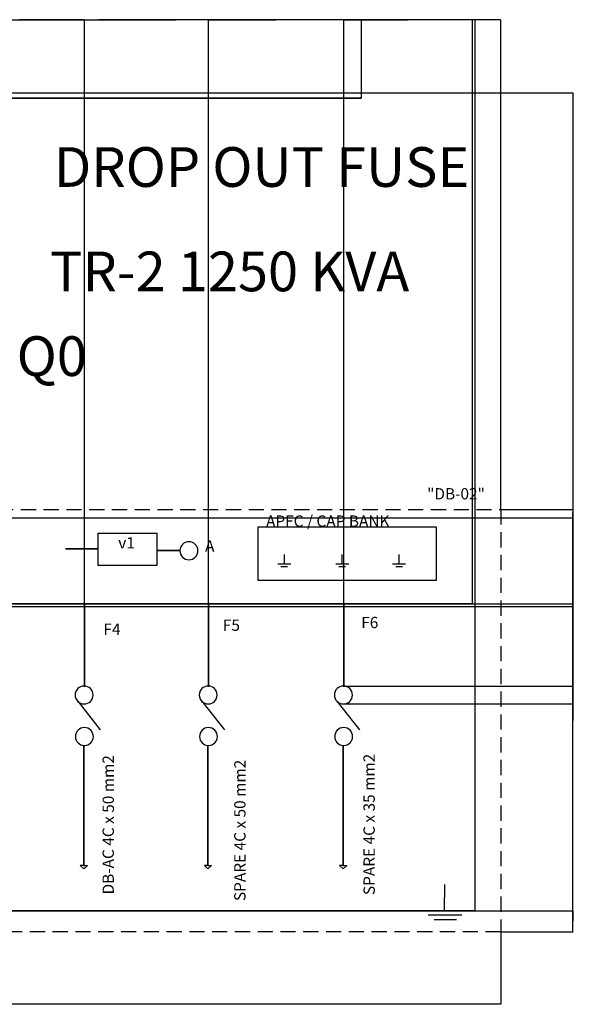
# Model space of a CAD drawing. Units: millimetres. Extents: x 1832 to 3146, y 927 to 1751.
# Tile 4 of 4: x 2683 to 3146, y 927 to 1751. Entities that reach past the tile are written whole.
import ezdxf

# ---------------------------------------------------------------- set-up
doc = ezdxf.new("R2010")
doc.units = ezdxf.units.MM
doc.header["$MEASUREMENT"] = 0
doc.linetypes.add('DASHED', pattern=[19.05, 12.7, -6.35])
doc.layers.get('0').update_dxf_attribs({"color": 2, "lineweight": 35})
doc.layers.get('0').transparency = 0.01
for name, color, linetype, lineweight in [('A-ANNO-DIMS', 2, 'Continuous', 18), ('E-ANNO-TEXT', 7, 'Continuous', 18), ('E-POWR-EQPM', 2, 'Continuous', 25), ('E-POWR-PNLS', 3, 'DASHED', 25), ('E-POWR-WIRE', 7, 'Continuous', 35)]:
    doc.layers.add(name, color=color, linetype=linetype, lineweight=lineweight)
doc.styles.get("Standard").update_dxf_attribs({"font": 'arial.ttf'})
doc.dimstyles.get("Standard").update_dxf_attribs({"dimtxt": 0.18, "dimasz": 0.18, "dimexe": 0.18, "dimexo": 0.0625, "dimgap": 0.09, "dimtad": 0, "dimtih": 1, "dimtoh": 1, "dimdec": 4, "dimzin": 0, "dimdsep": 46, "dimtxsty": 'Standard', "dimcen": 0.09, "dimadec": 0, "dimazin": 0, "dimtfac": 1, "dimtdec": 4, "dimtofl": 0, "dimtmove": 0, "dimatfit": 3, "dimfxl": 1, "dimtolj": 1, "dimtzin": 0, "dimarcsym": 0})

# ---------------------------------------------------------------- blocks, each defined once
blk = doc.blocks.new('CB-FEEDER')
blk.add_line((1982.97, 1178.23), (2001.83, 1154.39))
for points in [[(1980.83, 1183.48, 1), (1995.83, 1183.48, 1)], [(1981.05, 1148.75, 1), (1996.05, 1148.75, 1)]]:
    blk.add_lwpolyline(points, format="xyb", close=True)
blk = doc.blocks.new('CABLE-ARROW')
for p, q in [((1988.1, 1040.89), (1985.1, 1040.84)), ((1985.1, 1040.84), (1988.1, 1038.05)), ((1988.1, 1040.89), (1991.1, 1040.89)), ((1991.1, 1040.89), (1988.1, 1038.05))]:
    blk.add_line(p, q)
blk = doc.blocks.new('EARTH')
for p, q in [((2904.21, 1303.5), (2904.21, 1295.71)), ((2898.96, 1295.71), (2909.83, 1295.71)), ((2901.62, 1293.58), (2907.16, 1293.58))]:
    blk.add_line(p, q)
blk = doc.blocks.new('*D9')
at = {"layer": 'A-ANNO-DIMS', "color": 0, "lineweight": -2, "transparency": 16777216}
for p, q in [((1892.94, 1002.86), (1892.94, 927.26)), ((3085.33, 987.73), (3085.33, 927.26)), ((1893.12, 927.44), (2488.68, 927.44)), ((3085.15, 927.44), (2489.59, 927.44))]:
    blk.add_line(p, q, dxfattribs=at)
at = {"layer": 'A-ANNO-DIMS', "color": 0, "lineweight": 35, "transparency": 16777216}
for points in [[(1893.12, 927.47), (1893.12, 927.41), (1892.94, 927.44)], [(3085.15, 927.47), (3085.15, 927.41), (3085.33, 927.44)]]:
    blk.add_solid(points, dxfattribs=at)
at = {"layer": 'Defpoints', "color": 0, "lineweight": 35, "transparency": 16777216}
for p in [(1892.94, 1002.93), (3085.33, 987.79), (3085.33, 927.44)]:
    blk.add_point(p, dxfattribs=at)
at = {"layer": 'A-ANNO-DIMS', "color": 0, "transparency": 16777216, "insert": (2489.13, 927.44), "char_height": 0.18, "attachment_point": 5}
blk.add_mtext('\\A1;1192.4', dxfattribs=at)
blk = doc.blocks.new('*D10')
at = {"layer": 'A-ANNO-DIMS', "color": 0, "lineweight": -2, "transparency": 16777216}
for p, q in [((2658.48, 1689.58), (3145.86, 1689.58)), ((3145.68, 1689.4), (3145.68, 1338.87)), ((3145.68, 987.97), (3145.68, 1338.5)), ((3085.39, 987.79), (3145.86, 987.79))]:
    blk.add_line(p, q, dxfattribs=at)
at = {"layer": 'A-ANNO-DIMS', "color": 0, "lineweight": 35, "transparency": 16777216}
for points in [[(3145.65, 1689.4), (3145.71, 1689.4), (3145.68, 1689.58)], [(3145.65, 987.97), (3145.71, 987.97), (3145.68, 987.79)]]:
    blk.add_solid(points, dxfattribs=at)
at = {"layer": 'Defpoints', "color": 0, "lineweight": 35, "transparency": 16777216}
for p in [(2658.42, 1689.58), (3145.68, 1689.58), (3085.33, 987.79)]:
    blk.add_point(p, dxfattribs=at)
at = {"layer": 'A-ANNO-DIMS', "color": 0, "transparency": 16777216, "insert": (3145.68, 1338.68), "char_height": 0.18, "attachment_point": 5}
blk.add_mtext('\\A1;701.8', dxfattribs=at)
blk = doc.blocks.new('*D18')
at = {"layer": 'A-ANNO-DIMS', "color": 0, "lineweight": -2, "transparency": 16777216}
for p, q in [((2627.92, 1262.43), (2627.92, 1750.84)), ((2628.1, 1750.66), (2682.1, 1750.66)), ((2737.01, 1750.66), (2683.01, 1750.66)), ((2737.19, 1262.43), (2737.19, 1750.84))]:
    blk.add_line(p, q, dxfattribs=at)
at = {"layer": 'A-ANNO-DIMS', "color": 0, "lineweight": 35, "transparency": 16777216}
for points in [[(2628.1, 1750.69), (2628.1, 1750.63), (2627.92, 1750.66)], [(2737.01, 1750.69), (2737.01, 1750.63), (2737.19, 1750.66)]]:
    blk.add_solid(points, dxfattribs=at)
at = {"layer": 'Defpoints', "color": 0, "lineweight": 35, "transparency": 16777216}
for p in [(2737.19, 1750.66), (2627.92, 1262.37), (2737.19, 1262.37)]:
    blk.add_point(p, dxfattribs=at)
at = {"layer": 'A-ANNO-DIMS', "color": 0, "transparency": 16777216, "insert": (2682.56, 1750.66), "char_height": 0.18, "attachment_point": 5}
blk.add_mtext('\\A1;109.27', dxfattribs=at)
blk = doc.blocks.new('*D19')
at = {"layer": 'A-ANNO-DIMS', "color": 0, "lineweight": -2, "transparency": 16777216}
for p, q in [((2737.19, 1262.43), (2737.19, 1750.84)), ((2737.37, 1750.66), (2788.62, 1750.66)), ((2840.78, 1750.66), (2789.53, 1750.66)), ((2840.96, 1262.43), (2840.96, 1750.84))]:
    blk.add_line(p, q, dxfattribs=at)
at = {"layer": 'A-ANNO-DIMS', "color": 0, "lineweight": 35, "transparency": 16777216}
for points in [[(2737.37, 1750.69), (2737.37, 1750.63), (2737.19, 1750.66)], [(2840.78, 1750.69), (2840.78, 1750.63), (2840.96, 1750.66)]]:
    blk.add_solid(points, dxfattribs=at)
at = {"layer": 'Defpoints', "color": 0, "lineweight": 35, "transparency": 16777216}
for p in [(2840.96, 1750.66), (2737.19, 1262.37), (2840.96, 1262.37)]:
    blk.add_point(p, dxfattribs=at)
at = {"layer": 'A-ANNO-DIMS', "color": 0, "transparency": 16777216, "insert": (2789.08, 1750.66), "char_height": 0.18, "attachment_point": 5}
blk.add_mtext('\\A1;103.77', dxfattribs=at)
blk = doc.blocks.new('*D20')
at = {"layer": 'A-ANNO-DIMS', "color": 0, "lineweight": -2, "transparency": 16777216}
for p, q in [((2840.96, 1262.43), (2840.96, 1750.84)), ((2841.14, 1750.66), (2897.04, 1750.66)), ((2953.85, 1750.66), (2897.95, 1750.66)), ((2954.03, 1262.43), (2954.03, 1750.84))]:
    blk.add_line(p, q, dxfattribs=at)
at = {"layer": 'A-ANNO-DIMS', "color": 0, "lineweight": 35, "transparency": 16777216}
for points in [[(2841.14, 1750.69), (2841.14, 1750.63), (2840.96, 1750.66)], [(2953.85, 1750.69), (2953.85, 1750.63), (2954.03, 1750.66)]]:
    blk.add_solid(points, dxfattribs=at)
at = {"layer": 'Defpoints', "color": 0, "lineweight": 35, "transparency": 16777216}
for p in [(2954.03, 1750.66), (2840.96, 1262.37), (2954.03, 1262.37)]:
    blk.add_point(p, dxfattribs=at)
at = {"layer": 'A-ANNO-DIMS', "color": 0, "transparency": 16777216, "insert": (2897.49, 1750.66), "char_height": 0.18, "attachment_point": 5}
blk.add_mtext('\\A1;113.07', dxfattribs=at)
blk = doc.blocks.new('*D22')
at = {"layer": 'A-ANNO-DIMS', "color": 0, "lineweight": -2, "transparency": 16777216}
for p, q in [((3085.39, 1341.19), (3145.86, 1341.19)), ((3145.68, 1341.01), (3145.68, 1164.67)), ((3145.68, 987.97), (3145.68, 1164.31)), ((3085.39, 987.79), (3145.86, 987.79))]:
    blk.add_line(p, q, dxfattribs=at)
at = {"layer": 'A-ANNO-DIMS', "color": 0, "lineweight": 35, "transparency": 16777216}
for points in [[(3145.65, 1341.01), (3145.71, 1341.01), (3145.68, 1341.19)], [(3145.65, 987.97), (3145.71, 987.97), (3145.68, 987.79)]]:
    blk.add_solid(points, dxfattribs=at)
at = {"layer": 'Defpoints', "color": 0, "lineweight": 35, "transparency": 16777216}
for p in [(3085.33, 1341.19), (3145.68, 1341.19), (3085.33, 987.79)]:
    blk.add_point(p, dxfattribs=at)
at = {"layer": 'A-ANNO-DIMS', "color": 0, "transparency": 16777216, "insert": (3145.68, 1164.49), "char_height": 0.18, "attachment_point": 5}
blk.add_mtext('\\A1;353.4', dxfattribs=at)
blk = doc.blocks.new('*D26')
at = {"layer": 'A-ANNO-DIMS', "color": 0, "lineweight": -2, "transparency": 16777216}
for p, q in [((2417.38, 1341.25), (2417.38, 1750.84)), ((2417.56, 1750.66), (2750.89, 1750.66)), ((3085.15, 1750.66), (2751.82, 1750.66)), ((3085.33, 1341.25), (3085.33, 1750.84))]:
    blk.add_line(p, q, dxfattribs=at)
at = {"layer": 'A-ANNO-DIMS', "color": 0, "lineweight": 35, "transparency": 16777216}
for points in [[(2417.56, 1750.69), (2417.56, 1750.63), (2417.38, 1750.66)], [(3085.15, 1750.69), (3085.15, 1750.63), (3085.33, 1750.66)]]:
    blk.add_solid(points, dxfattribs=at)
at = {"layer": 'Defpoints', "color": 0, "lineweight": 35, "transparency": 16777216}
for p in [(3085.33, 1750.66), (2417.38, 1341.19), (3085.33, 1341.19)]:
    blk.add_point(p, dxfattribs=at)
at = {"layer": 'A-ANNO-DIMS', "color": 0, "transparency": 16777216, "insert": (2751.35, 1750.66), "char_height": 0.18, "attachment_point": 5}
blk.add_mtext('\\A1;667.94', dxfattribs=at)
blk = doc.blocks.new('*D28')
at = {"layer": 'A-ANNO-DIMS', "color": 0, "lineweight": -2, "transparency": 16777216}
for p, q in [((2433.56, 1005.45), (2433.56, 1750.84)), ((2433.74, 1750.66), (2748.28, 1750.66)), ((3063.74, 1750.66), (2749.21, 1750.66)), ((3063.92, 1005.45), (3063.92, 1750.84))]:
    blk.add_line(p, q, dxfattribs=at)
at = {"layer": 'A-ANNO-DIMS', "color": 0, "lineweight": 35, "transparency": 16777216}
for points in [[(2433.74, 1750.69), (2433.74, 1750.63), (2433.56, 1750.66)], [(3063.74, 1750.69), (3063.74, 1750.63), (3063.92, 1750.66)]]:
    blk.add_solid(points, dxfattribs=at)
at = {"layer": 'Defpoints', "color": 0, "lineweight": 35, "transparency": 16777216}
for p in [(3063.92, 1750.66), (2433.56, 1005.39), (3063.92, 1005.39)]:
    blk.add_point(p, dxfattribs=at)
at = {"layer": 'A-ANNO-DIMS', "color": 0, "transparency": 16777216, "insert": (2748.74, 1750.66), "char_height": 0.18, "attachment_point": 5}
blk.add_mtext('\\A1;630.36', dxfattribs=at)
blk = doc.blocks.new('*D31')
at = {"layer": 'A-ANNO-DIMS', "color": 0, "lineweight": -2, "transparency": 16777216}
for p, q in [((2954.03, 1262.43), (2954.03, 1750.84)), ((2954.21, 1750.66), (3007.49, 1750.66)), ((3061.65, 1750.66), (3008.37, 1750.66)), ((3061.83, 1262.43), (3061.83, 1750.84))]:
    blk.add_line(p, q, dxfattribs=at)
at = {"layer": 'A-ANNO-DIMS', "color": 0, "lineweight": 35, "transparency": 16777216}
for points in [[(2954.21, 1750.69), (2954.21, 1750.63), (2954.03, 1750.66)], [(3061.65, 1750.69), (3061.65, 1750.63), (3061.83, 1750.66)]]:
    blk.add_solid(points, dxfattribs=at)
at = {"layer": 'Defpoints', "color": 0, "lineweight": 35, "transparency": 16777216}
for p in [(3061.83, 1750.66), (2954.03, 1262.37), (3061.83, 1262.37)]:
    blk.add_point(p, dxfattribs=at)
at = {"layer": 'A-ANNO-DIMS', "color": 0, "transparency": 16777216, "insert": (3007.93, 1750.66), "char_height": 0.18, "attachment_point": 5}
blk.add_mtext('\\A1;107.81', dxfattribs=at)
blk = doc.blocks.new('*D33')
at = {"layer": 'A-ANNO-DIMS', "color": 0, "lineweight": -2, "transparency": 16777216}
for p, q in [((2659.21, 1685.57), (2659.21, 1750.84)), ((2659.39, 1750.66), (2813.63, 1750.66)), ((2968.8, 1750.66), (2814.56, 1750.66)), ((2968.98, 1685.38), (2968.98, 1750.84))]:
    blk.add_line(p, q, dxfattribs=at)
at = {"layer": 'A-ANNO-DIMS', "color": 0, "lineweight": 35, "transparency": 16777216}
for points in [[(2659.39, 1750.69), (2659.39, 1750.63), (2659.21, 1750.66)], [(2968.8, 1750.69), (2968.8, 1750.63), (2968.98, 1750.66)]]:
    blk.add_solid(points, dxfattribs=at)
at = {"layer": 'Defpoints', "color": 0, "lineweight": 35, "transparency": 16777216}
for p in [(2968.98, 1750.66), (2659.21, 1685.51), (2968.98, 1685.32)]:
    blk.add_point(p, dxfattribs=at)
at = {"layer": 'A-ANNO-DIMS', "color": 0, "transparency": 16777216, "insert": (2814.1, 1750.66), "char_height": 0.18, "attachment_point": 5}
blk.add_mtext('\\A1;309.76', dxfattribs=at)
blk = doc.blocks.new('*D46')
at = {"layer": 'A-ANNO-DIMS', "color": 0, "lineweight": -2, "transparency": 16777216}
for p, q in [((2953.87, 1193.48), (3145.86, 1193.48)), ((3145.68, 1193.3), (3145.68, 1186.16)), ((2953.87, 1178.48), (3145.86, 1178.48)), ((3145.68, 1178.66), (3145.68, 1185.8))]:
    blk.add_line(p, q, dxfattribs=at)
at = {"layer": 'A-ANNO-DIMS', "color": 0, "lineweight": 35, "transparency": 16777216}
for points in [[(3145.65, 1193.3), (3145.71, 1193.3), (3145.68, 1193.48)], [(3145.65, 1178.66), (3145.71, 1178.66), (3145.68, 1178.48)]]:
    blk.add_solid(points, dxfattribs=at)
at = {"layer": 'Defpoints', "color": 0, "lineweight": 35, "transparency": 16777216}
for p in [(2953.81, 1193.48), (2953.81, 1178.48), (3145.68, 1178.48)]:
    blk.add_point(p, dxfattribs=at)
at = {"layer": 'A-ANNO-DIMS', "color": 0, "transparency": 16777216, "insert": (3145.68, 1185.98), "char_height": 0.18, "attachment_point": 5}
blk.add_mtext('\\A1;15.00', dxfattribs=at)
blk = doc.blocks.new('*D47')
at = {"layer": 'A-ANNO-DIMS', "color": 0, "lineweight": -2, "transparency": 16777216}
for p, q in [((2330.79, 1334.1), (3145.86, 1334.1)), ((3145.68, 1333.92), (3145.68, 1297.17)), ((3145.68, 1260.06), (3145.68, 1296.81)), ((2311.47, 1259.88), (3145.86, 1259.88))]:
    blk.add_line(p, q, dxfattribs=at)
at = {"layer": 'A-ANNO-DIMS', "color": 0, "lineweight": 35, "transparency": 16777216}
for points in [[(3145.65, 1333.92), (3145.71, 1333.92), (3145.68, 1334.1)], [(3145.65, 1260.06), (3145.71, 1260.06), (3145.68, 1259.88)]]:
    blk.add_solid(points, dxfattribs=at)
at = {"layer": 'Defpoints', "color": 0, "lineweight": 35, "transparency": 16777216}
for p in [(2330.73, 1334.1), (2311.41, 1259.88), (3145.68, 1259.88)]:
    blk.add_point(p, dxfattribs=at)
at = {"layer": 'A-ANNO-DIMS', "color": 0, "transparency": 16777216, "insert": (3145.68, 1296.99), "char_height": 0.18, "attachment_point": 5}
blk.add_mtext('\\A1;74.22', dxfattribs=at)
blk = doc.blocks.new('*D48')
at = {"layer": 'A-ANNO-DIMS', "color": 0, "lineweight": -2, "transparency": 16777216}
for p, q in [((3085.39, 1341.19), (3145.86, 1341.19)), ((3145.68, 1341.01), (3145.68, 1301.96)), ((3145.68, 1262.55), (3145.68, 1301.6)), ((3061.9, 1262.37), (3145.86, 1262.37))]:
    blk.add_line(p, q, dxfattribs=at)
at = {"layer": 'A-ANNO-DIMS', "color": 0, "lineweight": 35, "transparency": 16777216}
for points in [[(3145.65, 1341.01), (3145.71, 1341.01), (3145.68, 1341.19)], [(3145.65, 1262.55), (3145.71, 1262.55), (3145.68, 1262.37)]]:
    blk.add_solid(points, dxfattribs=at)
at = {"layer": 'Defpoints', "color": 0, "lineweight": 35, "transparency": 16777216}
for p in [(3085.33, 1341.19), (3061.83, 1262.37), (3145.68, 1262.37)]:
    blk.add_point(p, dxfattribs=at)
at = {"layer": 'A-ANNO-DIMS', "color": 0, "transparency": 16777216, "insert": (3145.68, 1301.78), "char_height": 0.18, "attachment_point": 5}
blk.add_mtext('\\A1;78.82', dxfattribs=at)
blk = doc.blocks.new('*D49')
at = {"layer": 'A-ANNO-DIMS', "color": 0, "lineweight": -2, "transparency": 16777216}
for p, q in [((3063.98, 1005.39), (3145.86, 1005.39)), ((3145.68, 1005.21), (3145.68, 996.77)), ((3145.68, 987.97), (3145.68, 996.41)), ((3085.39, 987.79), (3145.86, 987.79))]:
    blk.add_line(p, q, dxfattribs=at)
at = {"layer": 'A-ANNO-DIMS', "color": 0, "lineweight": 35, "transparency": 16777216}
for points in [[(3145.65, 1005.21), (3145.71, 1005.21), (3145.68, 1005.39)], [(3145.65, 987.97), (3145.71, 987.97), (3145.68, 987.79)]]:
    blk.add_solid(points, dxfattribs=at)
at = {"layer": 'Defpoints', "color": 0, "lineweight": 35, "transparency": 16777216}
for p in [(3063.92, 1005.39), (3085.33, 987.79), (3145.68, 987.79)]:
    blk.add_point(p, dxfattribs=at)
at = {"layer": 'A-ANNO-DIMS', "color": 0, "transparency": 16777216, "insert": (3145.68, 996.59), "char_height": 0.18, "attachment_point": 5}
blk.add_mtext('\\A1;17.598', dxfattribs=at)

msp = doc.modelspace()

# ---------------------------------------------------------------- linework, layer by layer
at = {"layer": 'E-POWR-EQPM'}
for p, q in [((3038.3597, 1027.5619), (3038.1974, 1005.3868)), ((3024.733, 1002.1152), (3052.7975, 1002.1152)), ((3029.5997, 998.0632), (3048.4174, 998.0632))]:
    msp.add_line(p, q, dxfattribs=at)
for points in [[(2882.4379, 1326.7295), (3031.5065, 1326.7295), (3031.5065, 1281.8291), (2882.4379, 1281.8291)], [(2748.6078, 1321.4322), (2797.7683, 1321.4322), (2797.7683, 1294.2185), (2748.6078, 1294.2185)]]:
    msp.add_lwpolyline(points, close=True, dxfattribs=at)
msp.add_lwpolyline([(2817.124, 1306.6378, 1), (2832.124, 1306.6378, 1)], format="xyb", close=True, dxfattribs=at)
at = {"layer": 'E-POWR-PNLS'}
msp.add_lwpolyline([(2417.3834, 1341.189), (3085.3254, 1341.189), (3085.3254, 987.7892), (2417.3834, 987.7892)], close=True, dxfattribs=at)
at = {"layer": 'E-POWR-WIRE'}
for p, q in [((2063.171, 1685.3164), (2684.8145, 1685.3164)), ((2684.8145, 1685.3164), (2968.9766, 1685.3164)), ((2721.3701, 1308.1572), (2748.6078, 1308.1572)), ((2797.7683, 1306.8297), (2817.6983, 1306.8297)), ((2433.5628, 1262.3723), (2814.7999, 1262.3723)), ((2737.1914, 1262.3723), (2737.1914, 1192.7373)), ((2814.7999, 1262.3723), (3061.8349, 1262.3723)), ((2840.9604, 1262.3723), (2840.9604, 1192.7373)), ((2954.0268, 1262.3723), (2954.0268, 1192.7373)), ((2736.742, 1143.7615), (2736.742, 1043.3883)), ((2840.511, 1143.7615), (2840.511, 1043.3883)), ((2953.5774, 1143.7615), (2953.5774, 1043.3883)), ((2433.5628, 1005.3868), (3063.9193, 1005.3868))]:
    msp.add_line(p, q, dxfattribs=at)

# ---------------------------------------------------------------- block references
at = {"layer": 'E-POWR-EQPM'}
for name, p in [('EARTH', (0, 0)), ('EARTH', (48.3892, 0)), ('EARTH', (95.9787, 0)), ('CB-FEEDER', (748.6432, 2.4945)), ('CB-FEEDER', (852.4121, 2.4945)), ('CB-FEEDER', (965.4785, 2.4945)), ('CABLE-ARROW', (748.6432, 2.4945)), ('CABLE-ARROW', (852.4121, 2.4945)), ('CABLE-ARROW', (965.4785, 2.4945))]:
    msp.add_blockref(name, p, dxfattribs=at)

# ---------------------------------------------------------------- texts
at = {"layer": 'E-ANNO-TEXT'}
for s, height, p in [('DROP OUT FUSE', 33.205653, (2711.8114, 1611.001)), ('TR-2 1250 KVA', 33.205653, (2708.4134, 1523.6862)), ('Q0', 33.20565, (2680.5666, 1452.8178)), ('"DB-02"', 9.44797, (3023.7876, 1349.5648)), ('APFC / CAP BANK', 9.447971, (2889.0975, 1326.7295)), ('v1', 9.44797, (2765.5388, 1308.5457)), ('v1', 9.44797, (2765.5388, 1308.5457)), ('A', 9.448, (2838.1173, 1305.8546)), ('F4', 9.44797, (2753.1341, 1236.2356)), ('F5', 9.44797, (2852.9895, 1239.6368)), ('F6', 9.44797, (2968.731, 1241.9043))]:
    msp.add_text(s, height=height, dxfattribs=at).set_placement(p)
for s, p in [('DB-AC 4C x 50 mm2', (2761.8892, 1019.1535)), ('SPARE 4C x 50 mm2', (2871.9672, 1013.6519)), ('SPARE 4C x 35 mm2', (2980.0313, 1018.6589))]:
    msp.add_text(s, height=9.447971, rotation=90, dxfattribs=at).set_placement(p)

# ---------------------------------------------------------------- dimensions: what is measured, and where the dimension line sits
at = {"layer": 'A-ANNO-DIMS'}
for base, p1, p2, override, picture, middle in [((3085.3254, 1750.6609), (2417.3834, 1341.189), (3085.3254, 1341.189), {"dimdec": 2, "dimlfac": 1, "dimrnd": 0, "dimzin": 0, "dimdsep": 46, "dimlunit": 2}, '*D26', (2751.3544, 1750.6609)), ((3063.9193, 1750.6609), (2433.5628, 1005.3868), (3063.9193, 1005.3868), {"dimdec": 2, "dimlfac": 1, "dimrnd": 0, "dimzin": 0, "dimdsep": 46, "dimlunit": 2}, '*D28', (2748.741, 1750.6609)), ((2737.1914, 1750.6609), (2627.9202, 1262.3723), (2737.1914, 1262.3723), {"dimdec": 2, "dimlfac": 1, "dimrnd": 0, "dimzin": 0, "dimdsep": 46, "dimlunit": 2}, '*D18', (2682.5558, 1750.6609)), ((2968.9766, 1750.6609), (2659.2142, 1685.5074), (2968.9766, 1685.3164), {"dimdec": 2, "dimlfac": 1, "dimrnd": 0, "dimzin": 0, "dimdsep": 46, "dimlunit": 2}, '*D33', (2814.0954, 1750.6609)), ((2840.9604, 1750.6609), (2737.1914, 1262.3723), (2840.9604, 1262.3723), {"dimdec": 2, "dimlfac": 1, "dimrnd": 0, "dimzin": 0, "dimdsep": 46, "dimlunit": 2}, '*D19', (2789.0759, 1750.6609)), ((2954.0268, 1750.6609), (2840.9604, 1262.3723), (2954.0268, 1262.3723), {"dimdec": 2, "dimlfac": 1, "dimrnd": 0, "dimzin": 0, "dimdsep": 46, "dimlunit": 2}, '*D20', (2897.4936, 1750.6609)), ((3061.8349, 1750.6609), (2954.0268, 1262.3723), (3061.8349, 1262.3723), {"dimdec": 2, "dimlfac": 1, "dimrnd": 0, "dimzin": 0, "dimdsep": 46, "dimlunit": 2}, '*D31', (3007.9308, 1750.6609)), ((3085.3254, 927.4392), (1892.9387, 1002.9254), (3085.3254, 987.7892), {"dimdec": 1, "dimlfac": 1, "dimrnd": 0, "dimzin": 0, "dimdsep": 46, "dimlunit": 2}, '*D9', (2489.1321, 927.4392))]:
    dim = msp.add_linear_dim(base=base, p1=p1, p2=p2, dimstyle='Standard', override=override, dxfattribs=at)
    dim.commit()
    dim.dimension.update_dxf_attribs({"geometry": picture, "text_midpoint": middle})
for base, p1, p2, override, picture, middle in [((3145.6754, 1689.5787), (3085.3254, 987.7892), (2658.4196, 1689.5787), {"dimdec": 1, "dimlfac": 1, "dimrnd": 0, "dimzin": 0, "dimdsep": 46, "dimlunit": 2}, '*D10', (3145.6754, 1338.6839)), ((3145.6754, 1262.3723), (3085.3254, 1341.189), (3061.8349, 1262.3723), {"dimdec": 2, "dimlfac": 1, "dimrnd": 0, "dimzin": 0, "dimdsep": 46, "dimlunit": 2}, '*D48', (3145.6754, 1301.7807)), ((3145.6754, 1341.189), (3085.3254, 987.7892), (3085.3254, 1341.189), {"dimdec": 1, "dimlfac": 1, "dimrnd": 0, "dimzin": 0, "dimdsep": 46, "dimlunit": 2}, '*D22', (3145.6754, 1164.4891)), ((3145.6754, 1259.8778), (2330.7306, 1334.0963), (2311.4119, 1259.8778), {"dimdec": 2, "dimlfac": 1, "dimrnd": 0, "dimzin": 0, "dimdsep": 46, "dimlunit": 2}, '*D47', (3145.6754, 1296.9871)), ((3145.6754, 1178.4775), (2953.8078, 1193.4775), (2953.8078, 1178.4775), {"dimdec": 2, "dimlfac": 1, "dimrnd": 0, "dimzin": 0, "dimdsep": 46, "dimlunit": 2}, '*D46', (3145.6754, 1185.9775)), ((3145.6754, 987.7892), (3063.9193, 1005.3868), (3085.3254, 987.7892), {"dimdec": 3, "dimlfac": 1, "dimrnd": 0, "dimzin": 0, "dimdsep": 46, "dimlunit": 2}, '*D49', (3145.6754, 996.588))]:
    dim = msp.add_linear_dim(base=base, p1=p1, p2=p2, angle=90, dimstyle='Standard', override=override, dxfattribs=at)
    dim.commit()
    dim.dimension.update_dxf_attribs({"geometry": picture, "text_midpoint": middle})

doc.saveas('drawing.dxf')
